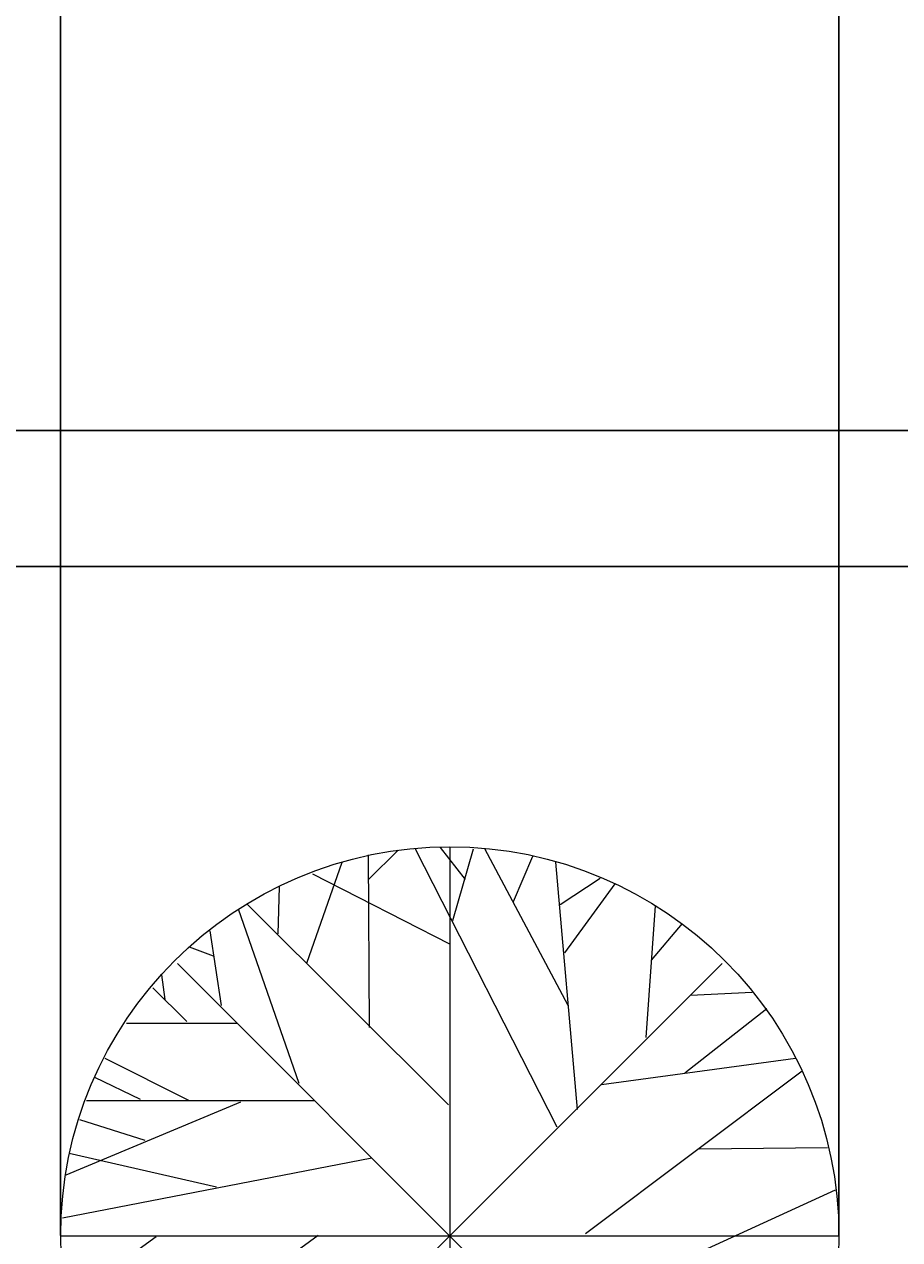
# Model space of a CAD drawing. Units: inches. Extents: x 2330 to 3943, y 1763 to 3461.
# Tile 38 of 40: x 3459 to 3594, y 2975 to 3163. Entities that reach past the tile are written whole.
import ezdxf

# ---------------------------------------------------------------- set-up
doc = ezdxf.new("R2010")
doc.units = ezdxf.units.IN
doc.layers.add('A-ANNO-DIMS', color=2, linetype='Continuous', lineweight=18)
doc.layers.add('L-PLNT', color=94, linetype='Continuous', lineweight=13)
doc.styles.get("Standard").update_dxf_attribs({"font": 'arial.ttf'})
doc.dimstyles.get("Standard").update_dxf_attribs({"dimtxt": 0.18, "dimasz": 0.18, "dimexe": 0.18, "dimexo": 0.0625, "dimgap": 0.09, "dimtad": 0, "dimtih": 1, "dimtoh": 1, "dimdec": 4, "dimzin": 0, "dimdsep": 46, "dimtxsty": 'Standard', "dimcen": 0.09, "dimadec": 0, "dimazin": 0, "dimtfac": 1, "dimtdec": 4, "dimtofl": 0, "dimtmove": 0, "dimatfit": 3, "dimfxl": 1, "dimtolj": 1, "dimtzin": 0, "dimarcsym": 0})

# ---------------------------------------------------------------- blocks, each defined once
blk = doc.blocks.new('*U14')
for p, q in [((0, 59.9996), (0, -60)), ((-12.5388, 54.9406), (-7.9613, 59.4546)), ((-12.3627, 32.1443), (-12.5388, 58.7776)), ((-5.3205, 59.6806), (16.5105, 16.7963)), ((2.426, 54.9406), (-1.4472, 59.9056)), ((0.4894, 48.6208), (3.6584, 59.6806)), ((18.2711, 35.5298), (5.419, 59.6806)), ((9.8203, 51.5549), (12.8133, 58.5516)), ((-22.0458, 42.0753), (-16.5881, 57.6486)), ((19.6795, 19.5047), (16.3344, 57.6486)), ((-21.1656, 55.8436), (-0.0388, 45.0094)), ((17.0387, 51.1035), (23.2006, 55.1666)), ((-26.4472, 46.5894), (-26.2712, 53.8116)), ((17.7429, 43.6552), (25.4894, 54.2636)), ((-31.2008, 51.1035), (-0.2149, 20.1818)), ((31.6513, 50.8778), (30.2429, 30.5643)), ((-32.6092, 50.4264), (-23.2782, 23.5674)), ((-37.0107, 47.0408), (-35.25, 35.5298)), ((31.1232, 42.5267), (35.8767, 48.1693)), ((-40.1797, 44.558), (-36.4825, 43.2038)), ((42, 42), (-42, -42)), ((42, -42), (-42, 42)), ((-43.8768, 36.4326), (-44.405, 40.2696)), ((-45.8134, 38.2383), (-40.5318, 33.0471)), ((37.1091, 37.1098), (46.6161, 37.5612)), ((36.2288, 25.1474), (48.9049, 35.0784)), ((-49.8627, 32.8214), (-32.7853, 32.8214)), ((-53.2078, 27.4044), (-40.1797, 20.859)), ((23.3767, 23.3417), (53.3063, 27.4044)), ((-54.7923, 24.4702), (-47.75, 21.0847)), ((54.3626, 25.3731), (20.9119, 0.3198)), ((-32.2571, 20.6333), (-59.1937, 9.348)), ((-56.0247, 20.859), (-20.8134, 20.859)), ((-57.081, 17.9248), (-47.0458, 14.7649)), ((38.5175, 13.4107), (58.2359, 13.6364)), ((-59.7219, 2.8025), (-12.0106, 12.0565)), ((-58.6656, 12.7336), (-35.9543, 7.5424)), ((29.3626, -6.6771), (59.4682, 7.091)), ((-54.6162, -24.7335), (-20.2853, 0.0941)), ((-60, 0), (60, 0)), ((-45.2853, -0.1316), (-59.0177, -10.0627)), ((9.2922, -9.1598), (59.6443, -2.8401)), ((-59.7219, -4.8714), (-54.2641, -6.6771)), ((-10.074, -10.0627), (-2.5036, -59.7178)), ((26.3697, -18.4138), (58.9401, -9.8369)), ((-58.4895, -12.3197), (-36.4825, -11.6426)), ((-53.2078, -27.442), (-16.7641, -16.6081)), ((-14.8275, -15.0282), (-14.6515, -57.6865)), ((-57.081, -18.4138), (-45.2853, -17.9624)), ((-52.6797, -18.188), (-55.4966, -22.0251)), ((18.6232, -18.6394), (26.7218, -53.3981)), ((18.7992, -18.6394), (57.3556, -17.2853)), ((38.1654, -18.188), (52.426, -29.0219)), ((-47.2219, -19.3166), (-50.2148, -26.3135)), ((-19.9331, -20.2194), (-28.5599, -52.721)), ((-0.0388, -19.0909), (25.8415, -53.8495)), ((-35.9543, -22.4765), (-44.0529, -40.5329)), ((45.9119, -24.0564), (55.595, -22.2508)), ((-38.9472, -29.0219), (-51.4472, -30.6018)), ((-46.5177, -30.1504), (-49.5106, -33.536)), ((30.419, -30.1504), (32.3556, -50.0125)), ((31.4753, -31.279), (49.6091, -33.3103)), ((-32.4331, -32.4075), (-48.1021, -35.5674)), ((-14.6515, -32.1818), (-3.912, -59.4922)), ((41.5105, -32.6332), (46.088, -38.0501)), ((-43.7008, -34.6645), (-46.6937, -37.373)), ((-14.6515, -36.2445), (-27.6797, -52.9467)), ((-6.2008, -36.2445), (17.919, -57.0094)), ((22.8485, -36.4702), (35.3485, -48.4326)), ((-24.6867, -37.8244), (-38.7712, -45.7241)), ((-26.2712, -43.9185), (-34.7219, -48.6583)), ((24.7852, -44.8213), (23.0246, -54.978)), ((-21.5177, -45.4984), (-19.9331, -56.1065)), ((5.9471, -46.6269), (10.5246, -58.5893)), ((-14.6515, -47.3041), (-25.0388, -54.3009)), ((-8.4895, -47.5298), (-11.4825, -58.5893)), ((-6.3768, -52.721), (-9.3698, -58.815)), ((8.4119, -53.1724), (3.8344, -59.4922))]:
    blk.add_line(p, q)
blk.add_circle((0, 0), 60)
blk = doc.blocks.new('*D69')
at = {"layer": 'A-ANNO-DIMS', "color": 0, "lineweight": -2, "transparency": 16777216}
for p, q in [((3464.39, 2975.89), (3464.39, 3461.3)), ((3464.57, 3461.12), (3524.11, 3461.12)), ((3584.21, 3461.12), (3524.67, 3461.12)), ((3584.39, 2975.89), (3584.39, 3461.3))]:
    blk.add_line(p, q, dxfattribs=at)
at = {"layer": 'A-ANNO-DIMS', "color": 0, "transparency": 16777216}
for points in [[(3464.57, 3461.15), (3464.57, 3461.09), (3464.39, 3461.12)], [(3584.21, 3461.15), (3584.21, 3461.09), (3584.39, 3461.12)]]:
    blk.add_solid(points, dxfattribs=at)
at = {"layer": 'Defpoints', "color": 0, "transparency": 16777216}
for p in [(3584.39, 3461.12), (3464.39, 2975.83), (3584.39, 2975.83)]:
    blk.add_point(p, dxfattribs=at)
at = {"layer": 'A-ANNO-DIMS', "color": 0, "transparency": 16777216, "insert": (3524.39, 3461.12), "char_height": 0.18, "attachment_point": 5}
blk.add_mtext('\\A1;120', dxfattribs=at)
blk = doc.blocks.new('*D86')
at = {"layer": 'A-ANNO-DIMS', "color": 0, "lineweight": -2, "transparency": 16777216}
for p, q in [((2979.18, 3100.04), (3942.54, 3100.04)), ((3942.36, 3099.86), (3942.36, 3089.72)), ((3942.36, 3079.22), (3942.36, 3089.36)), ((2979.18, 3079.04), (3942.54, 3079.04))]:
    blk.add_line(p, q, dxfattribs=at)
at = {"layer": 'A-ANNO-DIMS', "color": 0, "transparency": 16777216}
for points in [[(3942.33, 3099.86), (3942.39, 3099.86), (3942.36, 3100.04)], [(3942.33, 3079.22), (3942.39, 3079.22), (3942.36, 3079.04)]]:
    blk.add_solid(points, dxfattribs=at)
at = {"layer": 'Defpoints', "color": 0, "transparency": 16777216}
for p in [(2979.12, 3100.04), (2979.12, 3079.04), (3942.36, 3079.04)]:
    blk.add_point(p, dxfattribs=at)
at = {"layer": 'A-ANNO-DIMS', "color": 0, "transparency": 16777216, "insert": (3942.36, 3089.54), "char_height": 0.18, "attachment_point": 5}
blk.add_mtext('\\A1;21', dxfattribs=at)

msp = doc.modelspace()

# ---------------------------------------------------------------- block references
at = {"layer": 'L-PLNT'}
msp.add_blockref('*U14', (3524.3948, 2975.8319), dxfattribs=at)

# ---------------------------------------------------------------- dimensions: what is measured, and where the dimension line sits
at = {"layer": 'A-ANNO-DIMS'}
dim = msp.add_linear_dim(base=(3584.3948, 3461.1231), p1=(3464.3948, 2975.8319), p2=(3584.3948, 2975.8319), dimstyle='Standard', override={"dimdec": 0, "dimlfac": 1, "dimrnd": 0, "dimzin": 0, "dimdsep": 46, "dimlunit": 2}, dxfattribs=at)
dim.commit()
dim.dimension.update_dxf_attribs({"geometry": '*D69', "text_midpoint": (3524.3948, 3461.1231)})
dim = msp.add_linear_dim(base=(3942.361, 3079.0386), p1=(2979.1218, 3100.0386), p2=(2979.1218, 3079.0386), angle=90, dimstyle='Standard', override={"dimdec": 0, "dimlfac": 1, "dimrnd": 0, "dimzin": 0, "dimdsep": 46, "dimlunit": 2}, dxfattribs=at)
dim.commit()
dim.dimension.update_dxf_attribs({"geometry": '*D86', "text_midpoint": (3942.361, 3089.5386)})

doc.saveas('drawing.dxf')
